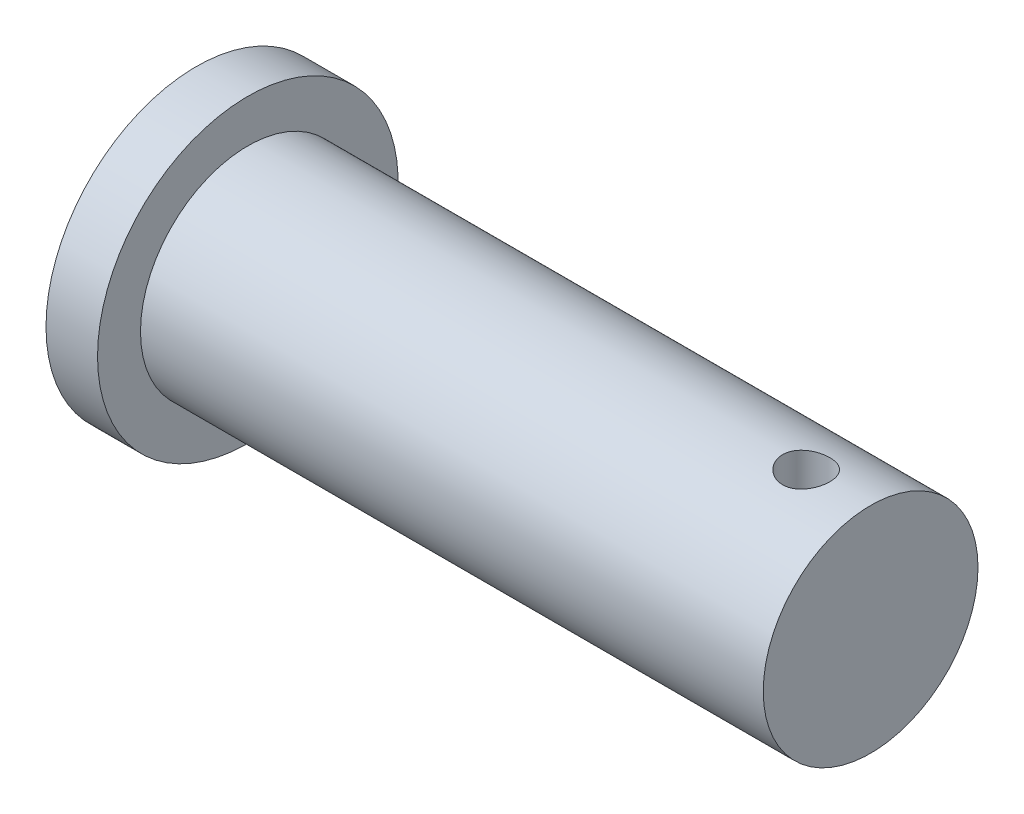
SolidWorks part; units mm, degrees
material "Plain Carbon Steel"
ref_plane "Front Plane" through (0, 0, 0) normal (0, 0, 1) x (1, 0, 0)
ref_plane "Top Plane" through (0, 0, 0) normal (0, 1, 0) x (1, 0, 0)
ref_plane "Right Plane" through (0, 0, 0) normal (1, 0, 0) x (0, 0, -1)
sketch "Pin Profile Sketch" plane through (0, 0, 0) normal (0, 0, 1) x (1, 0, 0)
  line L0 (0, 0) -> (0, 25)
  line L1 (0, 25) -> (-145, 25)
  line L2 (-145, 25) -> (-145, 35)
  line L3 (-145, 35) -> (-157, 35)
  line L4 (-157, 35) -> (-157, 0)
  line L5 (-157, 0) -> (0, 0)
  dimension "D1" = 12
  dimension "D2" = 35
  dimension "D3" = 25
  dimension "D4" = 157
revolve "Pin Body Revolve" add sketch "Pin Profile Sketch" angle 360 about L5
sketch "Split Pin Hole Sketch" plane through (0, 0, 0) normal (0, 1, 0) x (1, 0, 0)
  line L0 (-145, -35) -> (-145, 35) construction
  circle A0 centre (-15, 0) radius 5.4869
  dimension "D1" = 10.9739
  dimension "D2" = 130
extrude "Split Pin Hole Ø11" cut sketch "Split Pin Hole Sketch" against normal mid plane 60
